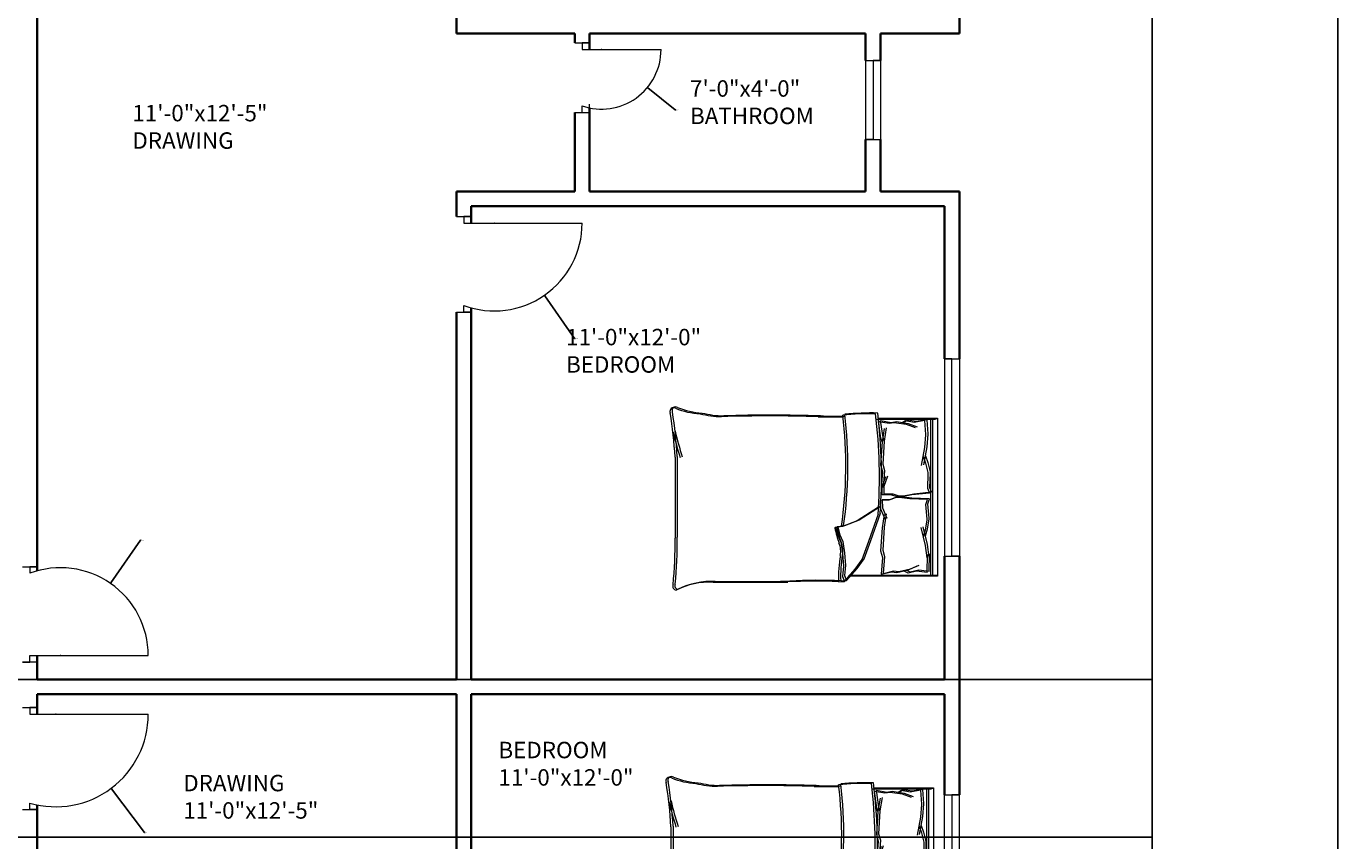
# Model space of a CAD drawing. Units: inches. Extents: x 2163 to 2982, y 1024 to 2288.
# Tile 19 of 22: x 2583 to 2982, y 1637 to 1885. Entities that reach past the tile are written whole.
import ezdxf

# ---------------------------------------------------------------- set-up
doc = ezdxf.new("R2010")
doc.units = ezdxf.units.IN
for name, color, linetype, lineweight in [('A-ANNO-DIMS', 2, 'Continuous', 18), ('A-ANNO-TTLB', 7, 'Continuous', 25), ('A-AREA-IDEN', 7, 'Continuous', 18), ('A-DOOR', 11, 'Continuous', 18), ('A-FURN', 8, 'Continuous', 13), ('A-GLAZ', 161, 'Continuous', 18), ('A-WALL', 7, 'Continuous', 35)]:
    doc.layers.add(name, color=color, linetype=linetype, lineweight=lineweight)
doc.styles.get("Standard").update_dxf_attribs({"font": 'arial.ttf'})
doc.dimstyles.get("Standard").update_dxf_attribs({"dimtxt": 0.18, "dimasz": 0.18, "dimexe": 0.18, "dimexo": 0.0625, "dimgap": 0.09, "dimtad": 0, "dimtih": 1, "dimtoh": 1, "dimdec": 4, "dimzin": 0, "dimdsep": 46, "dimtxsty": 'Standard', "dimcen": 0.09, "dimadec": 0, "dimazin": 0, "dimtfac": 1, "dimtdec": 4, "dimtofl": 0, "dimtmove": 0, "dimatfit": 3, "dimfxl": 1, "dimtolj": 1, "dimtzin": 0, "dimarcsym": 0})

# ---------------------------------------------------------------- blocks, each defined once
blk = doc.blocks.new('BED-DOUBLE')
for p, q in [((27.75, 52.87), (24.5, 49.16)), ((27.75, 52.87), (24.5, 49.16)), ((28.38, 53.1), (25.13, 49.39)), ((28.38, 53.1), (25.13, 49.39)), ((29.49, 52.95), (27.75, 52.87, 3.87)), ((29.49, 52.95), (27.75, 52.87, 3.87)), ((28.36, 51.33), (27.75, 52.87)), ((28.36, 51.33), (27.75, 52.87)), ((30.13, 53.18), (28.38, 53.1, 3.87)), ((29, 51.56), (28.38, 53.1)), ((30.13, 53.18), (28.38, 53.1, 3.87)), ((29, 51.56), (28.38, 53.1)), ((0, 51.49), (0.64, 51.49)), ((0, 3.47), (0, 51.49)), ((0, 51.27), (26.61, 51.27)), ((0, 51.27), (26.61, 51.27)), ((0.64, 51.49), (27.25, 51.49)), ((0.64, 51.49), (27.25, 51.49)), ((1.53, 3.48), (1.53, 51.27)), ((1.53, 3.47), (1.53, 51.27)), ((2.17, 3.7), (2.17, 51.49)), ((2.17, 3.7), (2.17, 51.49)), ((2.56, 50.11), (2.46, 44.71)), ((2.56, 50.11), (2.46, 44.71)), ((2.56, 50.11), (5.77, 49.73)), ((2.56, 50.11), (5.77, 49.73)), ((3.2, 50.34), (3.1, 44.94)), ((3.2, 50.34), (3.1, 44.94)), ((3.2, 50.34), (6.41, 49.96)), ((3.2, 50.34), (6.41, 49.96)), ((8.26, 49.31), (5.58, 48.13)), ((8.26, 49.31), (5.58, 48.13)), ((5.77, 49.73), (8.34, 50.33)), ((5.77, 49.73), (8.34, 50.33)), ((8.9, 49.54), (6.22, 48.36)), ((8.9, 49.54), (6.22, 48.36)), ((6.41, 49.96), (8.98, 50.56)), ((6.41, 49.96), (8.98, 50.56)), ((11.83, 50.11), (8.26, 49.31)), ((11.83, 50.11), (8.26, 49.31)), ((8.34, 50.33), (9.38, 49.81)), ((8.34, 50.33), (9.38, 49.81)), ((12.47, 50.34), (8.9, 49.54)), ((12.47, 50.34), (8.9, 49.54)), ((8.98, 50.56), (10.02, 50.04)), ((8.98, 50.56), (10.02, 50.04)), ((13.43, 49.92), (11.83, 50.11)), ((13.43, 49.92), (11.83, 50.11)), ((14.07, 50.15), (12.47, 50.34)), ((14.07, 50.15), (12.47, 50.34)), ((16.57, 50.7), (13.43, 49.92)), ((16.57, 50.7), (13.43, 49.92)), ((17.21, 50.93), (14.07, 50.15)), ((17.21, 50.93), (14.07, 50.15)), ((16.17, 45.57), (16.57, 50.7)), ((16.17, 45.57), (16.57, 50.7)), ((16.81, 45.79), (17.21, 50.93)), ((16.81, 45.79), (17.21, 50.93)), ((24.5, 49.16), (22.33, 46.22)), ((24.5, 49.16), (22.33, 46.22)), ((25.13, 49.39), (22.97, 46.45)), ((25.13, 49.39), (22.97, 46.45)), ((28.06, 48.23), (28.36, 51.33)), ((28.06, 48.23), (28.36, 51.33)), ((28.36, 44.36), (28.06, 48.23)), ((28.36, 44.36), (28.06, 48.23)), ((28.69, 48.46), (29, 51.56)), ((28.69, 48.46), (29, 51.56)), ((29, 44.59), (28.69, 48.46)), ((29, 44.59), (28.69, 48.46)), ((2.46, 44.71), (2.54, 45.71)), ((2.46, 44.71), (2.54, 45.71)), ((2.54, 45.71), (3.07, 41.91)), ((2.54, 45.71), (3.07, 41.91)), ((3.1, 44.94), (3.18, 45.94)), ((3.1, 44.94), (3.18, 45.94)), ((3.18, 45.94), (3.71, 42.14)), ((3.18, 45.94), (3.71, 42.14)), ((16.73, 43.61), (16.17, 45.57)), ((16.73, 43.61), (16.17, 45.57)), ((17.37, 43.83), (16.81, 45.79)), ((17.37, 43.83), (16.81, 45.79)), ((22.33, 46.22), (20.32, 40.64)), ((22.33, 46.22), (20.32, 40.64)), ((22.97, 46.45), (20.96, 40.87)), ((22.97, 46.45), (20.96, 40.87)), ((28.83, 40.95), (28.36, 44.36)), ((28.83, 40.95), (28.36, 44.36)), ((29.47, 41.18), (29, 44.59)), ((29.47, 41.18), (29, 44.59)), ((3.07, 41.91), (4.42, 36.49)), ((3.07, 41.91), (4.42, 36.49)), ((3.71, 42.14), (5.06, 36.72)), ((3.71, 42.14), (5.06, 36.72)), ((16.29, 36.6), (16.73, 43.61)), ((16.29, 36.6), (16.73, 43.61)), ((16.93, 36.82), (17.37, 43.83)), ((16.93, 36.82), (17.37, 43.83)), ((20.32, 40.64), (17.38, 32.31)), ((20.32, 40.64), (17.38, 32.31)), ((20.96, 40.87), (18.02, 32.53)), ((20.96, 40.87), (18.02, 32.53)), ((29.76, 38.94), (28.83, 40.95)), ((29.76, 38.94), (28.83, 40.95)), ((30.4, 39.17), (29.47, 41.18)), ((30.4, 39.17), (29.47, 41.18)), ((79.88, 15.29), (79.88, 39.91)), ((79.88, 15.29), (79.88, 39.91)), ((3.08, 37.14), (2.54, 34.2)), ((3.08, 37.13), (2.54, 34.2)), ((3.67, 39.2), (3.08, 37.14)), ((3.67, 39.2), (3.08, 37.13)), ((3.72, 37.36), (3.18, 34.43)), ((3.72, 37.36), (3.18, 34.43)), ((4.31, 39.43), (3.72, 37.36)), ((4.31, 39.43), (3.72, 37.36)), ((15.63, 32.56), (16.29, 36.6)), ((15.63, 32.56), (16.29, 36.6)), ((16.27, 32.79), (16.93, 36.82)), ((16.27, 32.79), (16.93, 36.82)), ((23.88, 34.45), (28.36, 36.15)), ((23.88, 34.45), (28.36, 36.15)), ((24.52, 34.68), (29, 36.38)), ((24.52, 34.68), (29, 36.38)), ((28.36, 36.15), (30.38, 36.46)), ((28.36, 36.15), (30.38, 36.46)), ((29, 36.38), (31.02, 36.69)), ((29, 36.38), (31.02, 36.69)), ((30.38, 36.46), (29.76, 38.94)), ((30.38, 36.46), (29.76, 38.94)), ((31.02, 36.69), (30.4, 39.17)), ((31.02, 36.69), (30.4, 39.17)), ((79.24, 15.06), (79.24, 39.68)), ((79.24, 15.06), (79.24, 39.68)), ((2.54, 34.2), (2.56, 33.88)), ((2.54, 34.2), (2.56, 33.88)), ((2.56, 33.88), (2.98, 29.46)), ((2.56, 33.88), (2.98, 29.46)), ((3.18, 34.43), (3.2, 34.11)), ((3.18, 34.43), (3.2, 34.11)), ((3.2, 34.11), (3.62, 29.68)), ((3.2, 34.11), (3.62, 29.68)), ((16.74, 30.75), (15.45, 33.82)), ((16.74, 30.75), (15.45, 33.82)), ((17.38, 30.98), (16.09, 34.05)), ((17.38, 30.98), (16.09, 34.05)), ((17.38, 30.26), (23.88, 34.45)), ((17.38, 30.26), (23.88, 34.45)), ((18.02, 30.49), (24.52, 34.68)), ((18.02, 30.49), (24.52, 34.68)), ((2.98, 29.46), (2.49, 27.98)), ((2.98, 29.46), (2.49, 27.98)), ((2.49, 27.98), (7.87, 27.73)), ((2.49, 27.98), (7.87, 27.73)), ((3.62, 29.68), (3.13, 28.21)), ((3.62, 29.68), (3.13, 28.2)), ((3.13, 28.21), (8.51, 27.96)), ((3.13, 28.2), (8.51, 27.96)), ((8.51, 27.96), (11.72, 27.58)), ((8.51, 27.96), (11.72, 27.58)), ((12.38, 27.44), (14.22, 28.13)), ((12.38, 27.44), (14.22, 28.13)), ((13.02, 27.66), (14.86, 28.36)), ((13.02, 27.66), (14.86, 28.36)), ((14.22, 28.13), (16.89, 28.3)), ((14.22, 28.13), (16.89, 28.3)), ((14.86, 28.36), (17.53, 28.53)), ((14.86, 28.36), (17.53, 28.53)), ((16.89, 28.3), (16.74, 30.75)), ((16.89, 28.3), (16.74, 30.75)), ((17.53, 28.53), (17.38, 30.98)), ((17.53, 28.53), (17.38, 30.98)), ((1.87, 25.98), (7.22, 26.56)), ((1.87, 25.98), (7.22, 26.56)), ((2.45, 24.54), (1.87, 25.98)), ((2.45, 24.54), (1.87, 25.98)), ((2.3, 20.09), (2.45, 24.54)), ((2.3, 20.09), (2.45, 24.54)), ((2.51, 26.21), (7.86, 26.79)), ((2.51, 26.21), (7.86, 26.79)), ((3.09, 24.77), (2.51, 26.21)), ((3.09, 24.77), (2.51, 26.21)), ((2.94, 20.32), (3.09, 24.77)), ((2.94, 20.32), (3.09, 24.77)), ((7.22, 26.56), (10.4, 27.14)), ((7.22, 26.56), (10.4, 27.14)), ((7.86, 26.79), (11.04, 27.37)), ((7.86, 26.79), (11.04, 27.37)), ((7.87, 27.73), (11.08, 27.35)), ((7.87, 27.73), (11.08, 27.35)), ((10.4, 27.14), (11.7, 27.14)), ((10.4, 27.14), (11.7, 27.14)), ((11.04, 27.37), (12.34, 27.37)), ((11.04, 27.37), (12.34, 27.37)), ((11.08, 27.35), (12.38, 27.44)), ((11.08, 27.35), (12.38, 27.44)), ((11.7, 27.14), (13.58, 26.56)), ((11.7, 27.14), (13.58, 26.56)), ((11.72, 27.58), (13.02, 27.66)), ((11.72, 27.58), (13.02, 27.66)), ((12.34, 27.37), (14.22, 26.79)), ((12.34, 27.37), (14.22, 26.79)), ((13.58, 26.56), (16.26, 26.56)), ((13.58, 26.56), (16.26, 26.56)), ((14.22, 26.79), (16.9, 26.79)), ((14.22, 26.79), (16.9, 26.79)), ((16.26, 24.1), (15.17, 20.96)), ((16.26, 24.1), (15.17, 20.96)), ((16.9, 24.33), (15.81, 21.19)), ((16.9, 24.33), (15.81, 21.19)), ((16.17, 19.38), (16.57, 24.52)), ((16.17, 19.38), (16.57, 24.52)), ((16.26, 26.56), (16.26, 24.1)), ((16.26, 26.56), (16.26, 24.1)), ((16.81, 19.61), (17.21, 24.74)), ((16.81, 19.61), (17.21, 24.74)), ((16.9, 26.79), (16.9, 24.33)), ((16.9, 26.79), (16.9, 24.33)), ((2.3, 19.77), (2.3, 20.09)), ((2.3, 19.77), (2.3, 20.09)), ((2.94, 20), (2.94, 20.32)), ((2.94, 20), (2.94, 20.32)), ((3.67, 17.11), (2.94, 20)), ((3.67, 17.11), (2.94, 20)), ((3.03, 16.88), (2.3, 19.77)), ((3.03, 16.88), (2.3, 19.77)), ((3.75, 14.85), (3.03, 16.88)), ((3.75, 14.85), (3.03, 16.88)), ((3.32, 12.11), (4.33, 17.6)), ((3.32, 12.11), (4.33, 17.6)), ((4.39, 15.08), (3.67, 17.11)), ((4.39, 15.08), (3.67, 17.11)), ((3.96, 12.34), (4.97, 17.83)), ((3.96, 12.34), (4.97, 17.83)), ((16.73, 17.42), (16.17, 19.38)), ((16.73, 17.42), (16.17, 19.38)), ((16.29, 10.41), (16.73, 17.42)), ((16.29, 10.41), (16.73, 17.42)), ((17.37, 17.65), (16.81, 19.61)), ((17.37, 17.65), (16.81, 19.61)), ((16.93, 10.64), (17.37, 17.65)), ((16.93, 10.64), (17.37, 17.65)), ((3.03, 8.28), (3.32, 12.11)), ((3.03, 8.28), (3.32, 12.11)), ((3.67, 8.51), (3.96, 12.34)), ((3.67, 8.51), (3.96, 12.34)), ((3.01, 8.18), (3.03, 8.28)), ((3.01, 8.18), (3.03, 8.28)), ((3.34, 3.9), (3.01, 8.18)), ((3.34, 3.9), (3.01, 8.18)), ((3.65, 8.41), (3.67, 8.51)), ((3.65, 8.41), (3.67, 8.51)), ((3.98, 4.13), (3.65, 8.41)), ((3.98, 4.13), (3.65, 8.41)), ((15.63, 6.38), (16.29, 10.41)), ((15.63, 6.38), (16.29, 10.41)), ((16.27, 6.61), (16.93, 10.64)), ((16.27, 6.61), (16.93, 10.64)), ((16.29, 10.41), (16.62, 9.28)), ((16.29, 10.41), (16.62, 9.28)), ((16.62, 9.28), (17.34, 4.18)), ((16.62, 9.28), (17.34, 4.18)), ((16.93, 10.64), (17.26, 9.51)), ((16.93, 10.64), (17.26, 9.51)), ((17.26, 9.51), (17.98, 4.41)), ((17.26, 9.51), (17.98, 4.41)), ((3.32, 3.89), (6.5, 4.47)), ((3.32, 3.89), (6.5, 4.47)), ((3.96, 4.12), (7.14, 4.7)), ((3.96, 4.12), (7.14, 4.7)), ((8.95, 5.05), (6.21, 6.06)), ((8.95, 5.05), (6.21, 6.06)), ((6.5, 4.47), (9.1, 4.04)), ((6.5, 4.47), (9.1, 4.04)), ((9.59, 5.28), (6.85, 6.29)), ((9.59, 5.28), (6.85, 6.29)), ((7.14, 4.7), (9.74, 4.27)), ((7.14, 4.7), (9.74, 4.27)), ((12.57, 4.47), (8.95, 5.05)), ((12.57, 4.47), (8.95, 5.05)), ((9.1, 4.04), (10.11, 4.62)), ((9.1, 4.04), (10.11, 4.62)), ((13.21, 4.7), (9.59, 5.28)), ((13.21, 4.7), (9.59, 5.28)), ((9.74, 4.27), (10.75, 4.85)), ((9.74, 4.27), (10.75, 4.85)), ((14.16, 4.76), (12.57, 4.47)), ((14.16, 4.76), (12.57, 4.47)), ((14.8, 4.99), (13.21, 4.7)), ((14.8, 4.99), (13.21, 4.7)), ((17.34, 4.18), (14.16, 4.76)), ((17.34, 4.18), (14.16, 4.76)), ((17.98, 4.41), (14.8, 4.99)), ((17.98, 4.41), (14.8, 4.99)), ((18.11, 3.48), (0, 3.48)), ((18.11, 3.47), (0, 3.47)), ((18.75, 3.7), (0.64, 3.7)), ((18.75, 3.7), (0.64, 3.7))]:
    blk.add_line(p, q)
for centre, radius, start, end in [((-6.66, 51.33), 36.18, 349.8763, 2.5657), ((-6.66, 51.33), 36.18, 349.8763, 2.5657), ((36.31, 182.27), 129.5, 266.9791, 273.8365), ((36.31, 182.27), 129.5, 266.9791, 273.8365), ((-6.02, 51.56), 36.18, 349.8763, 2.5657), ((-6.02, 51.56), 36.18, 349.8763, 2.5657), ((36.95, 182.49), 129.5, 266.9791, 273.8365), ((36.95, 182.49), 129.5, 266.9791, 273.8365), ((67.82, -4508.74), 4561.86, 90.00217, 90.28689), ((67.82, -4508.74), 4561.86, 90.00217, 90.28689), ((68.46, -4508.52), 4561.86, 90.00217, 90.28689), ((68.46, -4508.52), 4561.86, 90.00217, 90.28689), ((68.67, 76.16), 23.07, 267.4714, 296.4681), ((68.67, 76.16), 23.07, 267.4714, 296.4681), ((69.31, 76.39), 23.07, 267.4714, 296.4681), ((69.31, 76.39), 23.07, 267.4714, 296.4681), ((78.87, 54.41), 1.1, 332.6588, 86.02), ((78.87, 54.41), 1.1, 332.6588, 86.02), ((212.28, 41.15), 133.04, 174.4998, 180.6351), ((212.28, 41.15), 133.04, 174.4998, 180.6351), ((79.51, 54.64), 1.1, 332.6588, 86.02), ((79.51, 54.64), 1.1, 332.6588, 86.02), ((212.92, 41.38), 133.04, 174.4998, 180.6351), ((212.92, 41.38), 133.04, 174.4998, 180.6351), ((35.07, 43.74), 6.22, 168.6608, 203.7384), ((35.07, 43.74), 6.22, 168.6608, 203.7384), ((35.71, 43.97), 6.22, 168.6608, 203.7384), ((35.71, 43.97), 6.22, 168.6608, 203.7384), ((1.48, 31.15), 29.65, 10.6617, 19.8806), ((1.48, 31.15), 29.65, 10.6617, 19.8806), ((2.12, 31.38), 29.65, 10.6617, 19.8806), ((2.12, 31.38), 29.65, 10.6617, 19.8806), ((156.32, 17.76), 129.02, 171.7845, 186.9006), ((156.32, 17.76), 129.02, 171.7845, 186.9006), ((156.96, 17.98), 129.02, 171.7845, 186.9006), ((156.96, 17.98), 129.02, 171.7845, 186.9006), ((30.44, 36.64), 0.185, 250.2464, 1.1377), ((30.44, 36.64), 0.185, 250.2464, 1.1377), ((31.08, 36.86), 0.185, 250.2464, 1.1377), ((31.08, 36.86), 0.185, 250.2464, 1.1377), ((182.05, 21.36), 164.97, 176.0865, 186.7821), ((182.05, 21.36), 164.97, 176.0865, 186.7821), ((182.69, 21.59), 164.97, 176.0865, 186.7821), ((182.69, 21.59), 164.97, 176.0865, 186.7821), ((-23.71, -17.22), 106.46, 13.3832, 17.7053), ((-23.71, -17.22), 106.46, 13.3832, 17.7053), ((-23.07, -16.99), 106.46, 13.3832, 17.7053), ((-23.07, -16.99), 106.46, 13.3832, 17.7053), ((200.84, 21.43), 121.76, 182.9958, 189.4091), ((200.84, 21.43), 121.76, 182.9958, 189.4091), ((201.48, 21.66), 121.76, 182.9958, 189.4091), ((201.48, 21.65), 121.76, 182.9958, 189.4091), ((20.1, 85.16), 83.31, 268.7218, 275.604), ((20.1, 85.16), 83.31, 268.7218, 275.604), ((20.74, 85.39), 83.31, 268.7218, 275.604), ((20.74, 85.39), 83.31, 268.7218, 275.604), ((31.17, -167.31), 170.11, 88.4762, 91.0082), ((31.17, -167.31), 170.11, 88.4762, 91.0082), ((31.81, -167.08), 170.11, 88.4762, 91.0082), ((31.81, -167.08), 170.11, 88.4762, 91.0082), ((50.61, 484.82), 482.31, 268.2277, 271.7185), ((50.61, 484.82), 482.31, 268.2277, 271.7185), ((51.25, 485.05), 482.31, 268.2277, 271.7185), ((51.25, 485.05), 482.31, 268.2277, 271.7185), ((64.51, -26.9), 29.63, 76.0648, 88.9113), ((64.51, -26.9), 29.63, 76.0648, 88.9113), ((65.15, -26.67), 29.63, 76.0648, 88.9113), ((65.15, -26.67), 29.63, 76.0648, 88.9113), ((70.28, -21.66), 23.56, 67.9751, 86.652), ((70.28, -21.66), 23.56, 67.9751, 86.652), ((70.91, -21.43), 23.56, 67.9751, 86.652), ((70.91, -21.43), 23.56, 67.9751, 86.652), ((79.72, 1.09), 1.09, 236.1736, 23.4781), ((79.72, 1.09), 1.09, 236.1736, 23.4781), ((80.36, 1.32), 1.09, 236.1736, 23.4781), ((80.36, 1.32), 1.09, 236.1736, 23.4781)]:
    blk.add_arc(centre, radius, start, end)
blk = doc.blocks.new('WIN-24')
for p, q in [((0, 24), (4.5, 24)), ((0, 24), (0, 0)), ((4.5, 24), (2.25, 24)), ((2.25, 24), (2.25, 0)), ((4.5, 24), (4.5, 0)), ((2.25, 0), (0, 0)), ((0, 0), (4.5, 0))]:
    blk.add_line(p, q)
blk = doc.blocks.new('WIN-60')
for p, q in [((2.25, 60), (0, 60)), ((0, 60), (4.5, 60)), ((0, 60), (0, 0)), ((2.25, 0), (2.25, 60)), ((4.5, 60), (4.5, 0)), ((0, 0), (4.5, 0)), ((4.5, 0), (2.25, 0))]:
    blk.add_line(p, q)
blk = doc.blocks.new('*D29')
at = {"layer": 'A-ANNO-DIMS', "color": 0, "lineweight": -2, "transparency": 16777216}
for p, q in [((2285.34, 1738.83), (2285.34, 2288.1)), ((2285.52, 2287.92), (2576.05, 2287.92)), ((2867.16, 2287.92), (2576.63, 2287.92)), ((2867.34, 2229.33), (2867.34, 2288.1))]:
    blk.add_line(p, q, dxfattribs=at)
at = {"layer": 'A-ANNO-DIMS', "color": 0, "transparency": 16777216}
for points in [[(2285.52, 2287.95), (2285.52, 2287.89), (2285.34, 2287.92)], [(2867.16, 2287.95), (2867.16, 2287.89), (2867.34, 2287.92)]]:
    blk.add_solid(points, dxfattribs=at)
at = {"layer": 'Defpoints', "color": 0, "transparency": 16777216}
for p in [(2867.34, 2287.92), (2867.34, 2229.27), (2285.34, 1738.77)]:
    blk.add_point(p, dxfattribs=at)
at = {"layer": 'A-ANNO-DIMS', "color": 0, "transparency": 16777216, "insert": (2576.34, 2287.92), "char_height": 0.18, "attachment_point": 5}
blk.add_mtext('\\A1;582', dxfattribs=at)
blk = doc.blocks.new('*D31')
at = {"layer": 'A-ANNO-DIMS', "color": 0, "lineweight": -2, "transparency": 16777216}
for p, q in [((2867.4, 2229.27), (2926.17, 2229.27)), ((2925.99, 2229.09), (2925.99, 1957.95)), ((2925.99, 1686.45), (2925.99, 1957.59)), ((2862.9, 1686.27), (2926.17, 1686.27))]:
    blk.add_line(p, q, dxfattribs=at)
at = {"layer": 'A-ANNO-DIMS', "color": 0, "transparency": 16777216}
for points in [[(2925.96, 2229.09), (2926.02, 2229.09), (2925.99, 2229.27)], [(2925.96, 1686.45), (2926.02, 1686.45), (2925.99, 1686.27)]]:
    blk.add_solid(points, dxfattribs=at)
at = {"layer": 'Defpoints', "color": 0, "transparency": 16777216}
for p in [(2867.34, 2229.27), (2925.99, 2229.27), (2862.84, 1686.27)]:
    blk.add_point(p, dxfattribs=at)
at = {"layer": 'A-ANNO-DIMS', "color": 0, "transparency": 16777216, "insert": (2925.99, 1957.77), "char_height": 0.18, "attachment_point": 5}
blk.add_mtext('\\A1;543', dxfattribs=at)
blk = doc.blocks.new('*D32')
at = {"layer": 'A-ANNO-DIMS', "color": 0, "lineweight": -2, "transparency": 16777216}
for p, q in [((2867.4, 2229.27), (2926.17, 2229.27)), ((2925.99, 2229.09), (2925.99, 1686.35)), ((2925.99, 1143.25), (2925.99, 1685.99)), ((2867.4, 1143.07), (2926.17, 1143.07))]:
    blk.add_line(p, q, dxfattribs=at)
at = {"layer": 'A-ANNO-DIMS', "color": 0, "transparency": 16777216}
for points in [[(2925.96, 2229.09), (2926.02, 2229.09), (2925.99, 2229.27)], [(2925.96, 1143.25), (2926.02, 1143.25), (2925.99, 1143.07)]]:
    blk.add_solid(points, dxfattribs=at)
at = {"layer": 'Defpoints', "color": 0, "transparency": 16777216}
for p in [(2867.34, 2229.27), (2925.99, 2229.27), (2867.34, 1143.07)]:
    blk.add_point(p, dxfattribs=at)
at = {"layer": 'A-ANNO-DIMS', "color": 0, "transparency": 16777216, "insert": (2925.99, 1686.17), "char_height": 0.18, "attachment_point": 5}
blk.add_mtext('\\A1;1086.2', dxfattribs=at)
blk = doc.blocks.new('*D39')
at = {"layer": 'A-ANNO-DIMS', "color": 0, "lineweight": -2, "transparency": 16777216}
for p, q in [((2425.51, 1686.27), (2926.17, 1686.27)), ((2925.99, 1686.09), (2925.99, 1662.45)), ((2925.99, 1638.45), (2925.99, 1662.09)), ((2425.51, 1638.27), (2926.17, 1638.27))]:
    blk.add_line(p, q, dxfattribs=at)
at = {"layer": 'A-ANNO-DIMS', "color": 0, "transparency": 16777216}
for points in [[(2925.96, 1686.09), (2926.02, 1686.09), (2925.99, 1686.27)], [(2925.96, 1638.45), (2926.02, 1638.45), (2925.99, 1638.27)]]:
    blk.add_solid(points, dxfattribs=at)
at = {"layer": 'Defpoints', "color": 0, "transparency": 16777216}
for p in [(2425.44, 1686.27), (2925.99, 1686.27), (2425.44, 1638.27)]:
    blk.add_point(p, dxfattribs=at)
at = {"layer": 'A-ANNO-DIMS', "color": 0, "transparency": 16777216, "insert": (2925.99, 1662.27), "char_height": 0.18, "attachment_point": 5}
blk.add_mtext('\\A1;48', dxfattribs=at)
blk = doc.blocks.new('*D44')
at = {"layer": 'A-ANNO-DIMS', "color": 0, "lineweight": -2, "transparency": 16777216}
for p, q in [((2592.35, 1675.65), (2592.53, 1675.65)), ((2592.44, 1675.56), (2592.44, 1675.74)), ((2619.49, 1639.63), (2609.45, 1653)), ((2619.67, 1639.63), (2619.49, 1639.63))]:
    blk.add_line(p, q, dxfattribs=at)
at = {"layer": 'A-ANNO-DIMS', "color": 0, "transparency": 16777216}
blk.add_solid([(2609.48, 1653.02), (2609.43, 1652.98), (2609.34, 1653.14)], dxfattribs=at)
at = {"layer": 'Defpoints', "color": 0, "transparency": 16777216}
for p in [(2592.44, 1675.65), (2609.34, 1653.14)]:
    blk.add_point(p, dxfattribs=at)
at = {"layer": 'A-ANNO-DIMS', "color": 0, "transparency": 16777216, "insert": (2620.22, 1639.63), "char_height": 0.18, "attachment_point": 5}
blk.add_mtext('\\A1;R28.154', dxfattribs=at)
blk = doc.blocks.new('*D50')
at = {"layer": 'A-ANNO-DIMS', "color": 0, "lineweight": -2, "transparency": 16777216}
for p, q in [((2725.78, 1825.1), (2725.96, 1825.1)), ((2725.87, 1825.01), (2725.87, 1825.19)), ((2750.29, 1790.01), (2741.24, 1803.02)), ((2750.47, 1790.01), (2750.29, 1790.01))]:
    blk.add_line(p, q, dxfattribs=at)
at = {"layer": 'A-ANNO-DIMS', "color": 0, "transparency": 16777216}
blk.add_solid([(2741.26, 1803.04), (2741.21, 1803.01), (2741.13, 1803.17)], dxfattribs=at)
at = {"layer": 'Defpoints', "color": 0, "transparency": 16777216}
for p in [(2725.87, 1825.1), (2741.13, 1803.17)]:
    blk.add_point(p, dxfattribs=at)
at = {"layer": 'A-ANNO-DIMS', "color": 0, "transparency": 16777216, "insert": (2750.95, 1790.01), "char_height": 0.18, "attachment_point": 5}
blk.add_mtext('\\A1;R26.72', dxfattribs=at)
blk = doc.blocks.new('*D51')
at = {"layer": 'A-ANNO-DIMS', "color": 0, "lineweight": -2, "transparency": 16777216}
for p, q in [((2618.27, 1728.6), (2609.23, 1715.6)), ((2618.45, 1728.6), (2618.27, 1728.6)), ((2593.8, 1693.53), (2593.98, 1693.53)), ((2593.89, 1693.44), (2593.89, 1693.62))]:
    blk.add_line(p, q, dxfattribs=at)
at = {"layer": 'A-ANNO-DIMS', "color": 0, "transparency": 16777216}
blk.add_solid([(2609.21, 1715.62), (2609.26, 1715.58), (2609.13, 1715.45)], dxfattribs=at)
at = {"layer": 'Defpoints', "color": 0, "transparency": 16777216}
for p in [(2609.13, 1715.45), (2593.89, 1693.53)]:
    blk.add_point(p, dxfattribs=at)
at = {"layer": 'A-ANNO-DIMS', "color": 0, "transparency": 16777216, "insert": (2619, 1728.6), "char_height": 0.18, "attachment_point": 5}
blk.add_mtext('\\A1;R26.694', dxfattribs=at)
blk = doc.blocks.new('*D73')
at = {"layer": 'A-ANNO-DIMS', "color": 0, "lineweight": -2, "transparency": 16777216}
for p, q in [((2758.37, 1877.92), (2758.55, 1877.92)), ((2758.46, 1877.83), (2758.46, 1878.01)), ((2780.89, 1859.53), (2772.62, 1866.31)), ((2781.07, 1859.53), (2780.89, 1859.53))]:
    blk.add_line(p, q, dxfattribs=at)
at = {"layer": 'A-ANNO-DIMS', "color": 0, "transparency": 16777216}
blk.add_solid([(2772.64, 1866.34), (2772.6, 1866.29), (2772.48, 1866.43)], dxfattribs=at)
at = {"layer": 'Defpoints', "color": 0, "transparency": 16777216}
for p in [(2758.46, 1877.92), (2772.48, 1866.43)]:
    blk.add_point(p, dxfattribs=at)
at = {"layer": 'A-ANNO-DIMS', "color": 0, "transparency": 16777216, "insert": (2781.62, 1859.53), "char_height": 0.18, "attachment_point": 5}
blk.add_mtext('\\A1;R18.128', dxfattribs=at)

msp = doc.modelspace()

# ---------------------------------------------------------------- linework, layer by layer
at = {"layer": 'A-ANNO-TTLB'}
msp.add_lwpolyline([(2162.6841, 2274.6054), (2982.469, 2274.6054), (2982.469, 1045.9691), (2162.6841, 1045.9691)], close=True, dxfattribs=at)
at = {"layer": 'A-DOOR'}
for p, q in [((2750.3389, 1879.9188), (2754.8389, 1879.9188)), ((2754.8389, 1879.9188), (2752.5889, 1879.9188)), ((2752.5889, 1879.9188), (2752.5889, 1877.9188)), ((2752.5889, 1877.9188), (2776.5889, 1877.9188)), ((2752.5889, 1858.7688), (2752.5889, 1860.7688)), ((2754.8389, 1858.7688), (2754.8389, 1861.3385)), ((2750.3389, 1858.7688), (2754.8389, 1858.7688)), ((2714.3389, 1827.1014), (2718.8389, 1827.1014)), ((2718.8389, 1827.1014), (2716.5889, 1827.1014)), ((2716.5889, 1827.1014), (2716.5889, 1825.1014)), ((2716.5889, 1825.1014), (2752.5889, 1825.1014)), ((2716.5889, 1798.0467), (2716.5889, 1800.0467)), ((2714.3389, 1798.0467), (2718.8389, 1798.0467)), ((2718.8389, 1798.0467), (2716.5889, 1798.0467)), ((2582.3389, 1720.5499), (2586.8389, 1720.5499)), ((2586.8389, 1720.5499), (2584.5889, 1720.5499)), ((2584.5889, 1720.5499), (2584.5889, 1718.5499)), ((2584.5889, 1691.5305), (2584.5889, 1693.5305)), ((2584.5889, 1693.5305), (2620.5889, 1693.5305)), ((2586.8389, 1691.5305), (2582.3389, 1691.5305)), ((2582.3389, 1691.5305), (2584.5889, 1691.5305)), ((2582.3389, 1677.6524), (2586.8389, 1677.6524)), ((2586.8389, 1677.6524), (2584.5889, 1677.6524)), ((2584.5889, 1677.6524), (2584.5889, 1675.6524)), ((2584.5889, 1675.6524), (2620.5889, 1675.6524)), ((2584.5889, 1646.614), (2584.5889, 1648.614)), ((2582.3389, 1646.614), (2586.8389, 1646.614)), ((2586.8389, 1646.614), (2584.5889, 1646.614))]:
    msp.add_line(p, q, dxfattribs=at)
for centre, radius, start, end in [((2758.4614, 1877.9188), 18.1275, 251.097757, 360), ((2725.8704, 1825.1014), 26.7185, 249.672934, 360), ((2593.8949, 1693.5305), 26.694, 0, 110.402719), ((2592.4351, 1675.6524), 28.1538, 253.818042, 360)]:
    msp.add_arc(centre, radius, start, end, dxfattribs=at)
at = {"layer": 'A-WALL'}
for p, q in [((2586.8389, 2011.7688), (2586.8389, 1719.2751)), ((2714.3389, 1963.7688), (2714.3389, 1882.7688)), ((2867.3389, 1905.1374), (2867.3389, 1882.7688)), ((2714.3389, 1882.7688), (2750.3389, 1882.7688)), ((2750.3389, 1879.9188), (2750.3389, 1882.7688)), ((2838.8389, 1882.7688), (2754.8389, 1882.7688)), ((2754.8389, 1882.7688), (2754.8389, 1877.9188)), ((2754.8389, 1882.7688), (2838.8389, 1882.7688)), ((2838.8389, 1882.7688), (2838.8389, 1874.5615)), ((2867.3389, 1882.7688), (2843.3389, 1882.7688)), ((2843.3389, 1882.7688), (2862.8389, 1882.7688)), ((2843.3389, 1874.5615), (2843.3389, 1882.7688)), ((2754.8389, 1860.1569), (2754.8389, 1834.7688)), ((2750.3389, 1834.7688), (2750.3389, 1858.7688)), ((2838.8389, 1850.5615), (2838.8389, 1834.7688)), ((2843.3389, 1834.7688), (2843.3389, 1850.5615)), ((2714.3389, 1834.7688), (2750.3389, 1834.7688)), ((2714.3389, 1834.7688), (2714.3389, 1827.1014)), ((2754.8389, 1834.7688), (2838.8389, 1834.7688)), ((2843.3389, 1834.7688), (2867.3389, 1834.7688)), ((2867.3389, 1834.7688), (2867.3389, 1783.7638)), ((2718.8389, 1830.2688), (2862.8389, 1830.2688)), ((2718.8389, 1830.2688), (2718.8389, 1825.1014)), ((2862.8389, 1830.2688), (2862.8389, 1783.7638)), ((2714.3389, 1798.0467), (2714.3389, 1686.2688)), ((2718.8389, 1799.3247), (2718.8389, 1686.2688)), ((2862.8389, 1723.7638), (2862.8389, 1686.2688)), ((2867.3389, 1723.7638), (2867.3389, 1651.1733)), ((2586.8389, 1693.5305), (2586.8389, 1686.2688)), ((2586.8389, 1686.2688), (2714.3389, 1686.2688)), ((2718.8389, 1686.2688), (2862.8389, 1686.2688)), ((2586.8389, 1681.7688), (2714.3389, 1681.7688)), ((2586.8389, 1681.7688), (2586.8389, 1675.6524)), ((2714.3389, 1681.7688), (2714.3389, 1572.0744)), ((2718.8389, 1681.7688), (2718.8389, 1570.7042)), ((2718.8389, 1681.7688), (2862.8389, 1681.7688)), ((2862.8389, 1681.7688), (2862.8389, 1651.1733)), ((2586.8389, 1648.0603), (2586.8389, 1356.2688))]:
    msp.add_line(p, q, dxfattribs=at)

# ---------------------------------------------------------------- block references
at = {"layer": 'A-FURN', "rotation": 180}
for p in [(2860.7453, 1769.1724), (2859.4875, 1656.6782)]:
    msp.add_blockref('BED-DOUBLE', p, dxfattribs=at)
at = {"layer": 'A-GLAZ'}
for name, p in [('WIN-24', (2838.839, 1850.562)), ('WIN-60', (2862.839, 1723.7637))]:
    msp.add_blockref(name, p, dxfattribs=at)
at = {"layer": 'A-GLAZ', "extrusion": (0, 0, -1), "zscale": -1, "rotation": 180}
msp.add_blockref('WIN-60', (-2862.839, 1651.1734), dxfattribs=at)

# ---------------------------------------------------------------- texts
at = {"layer": 'A-AREA-IDEN', "char_height": 5, "attachment_point": 1}
for s, width, insert in [('7\'-0"x4\'-0"\\PBATHROOM', 37.624015, (2785.4074, 1868.576)), ('11\'-0"x12\'-5"\\PDRAWING', 86.750713, (2615.7616, 1861.0681)), ('11\'-0"x12\'-0"\\PBEDROOM', 49.776962, (2747.7027, 1792.9277)), ('BEDROOM\\P11\'-0"x12\'-0"', 60.332971, (2727.119, 1667.2605)), ('DRAWING\\P11\'-0"x12\'-5"', 69.474499, (2631.2335, 1657.2071))]:
    msp.add_mtext_dynamic_manual_height_columns(s, width=width, gutter_width=12.5, heights=[0], dxfattribs=dict(at, insert=insert))

# ---------------------------------------------------------------- dimensions: what is measured, and where the dimension line sits
at = {"layer": 'A-ANNO-DIMS'}
dim = msp.add_linear_dim(base=(2867.3389, 2287.9188), p1=(2285.3389, 1738.7688), p2=(2867.3389, 2229.2688), dimstyle='Standard', override={"dimdec": 0, "dimlfac": 1, "dimrnd": 0, "dimzin": 0, "dimdsep": 46, "dimlunit": 2}, dxfattribs=at)
dim.commit()
dim.dimension.update_dxf_attribs({"geometry": '*D29', "text_midpoint": (2576.3389, 2287.9188)})
for base, p1, p2, override, picture, middle in [((2925.9889, 2229.2688), (2862.8389, 1686.2688), (2867.3389, 2229.2688), {"dimdec": 0, "dimlfac": 1, "dimrnd": 0, "dimzin": 0, "dimdsep": 46, "dimlunit": 2}, '*D31', (2925.9889, 1957.7688)), ((2925.9889, 2229.2688), (2867.3389, 1143.0732), (2867.3389, 2229.2688), {"dimdec": 1, "dimlfac": 1, "dimrnd": 0, "dimzin": 0, "dimdsep": 46, "dimlunit": 2}, '*D32', (2925.9889, 1686.171)), ((2925.9889, 1686.2688), (2425.4434, 1638.2688), (2425.4434, 1686.2688), {"dimdec": 0, "dimlfac": 1, "dimrnd": 0, "dimzin": 0, "dimdsep": 46, "dimlunit": 2}, '*D39', (2925.9889, 1662.2688))]:
    dim = msp.add_linear_dim(base=base, p1=p1, p2=p2, angle=90, dimstyle='Standard', override=override, dxfattribs=at)
    dim.commit()
    dim.dimension.update_dxf_attribs({"geometry": picture, "text_midpoint": middle})
for center, mpoint, override, picture, middle in [((2758.4614, 1877.9188), (2772.4802, 1866.4262), {"dimdec": 3, "dimlfac": 1, "dimrnd": 0, "dimzin": 0, "dimdsep": 46, "dimlunit": 2}, '*D73', (2781.6214, 1859.5306)), ((2725.8704, 1825.1014), (2741.1329, 1803.1711), {"dimdec": 2, "dimlfac": 1, "dimrnd": 0, "dimzin": 0, "dimdsep": 46, "dimlunit": 2}, '*D50', (2750.9493, 1790.013)), ((2593.8949, 1693.5305), (2609.1288, 1715.4508), {"dimdec": 3, "dimlfac": 1, "dimrnd": 0, "dimzin": 0, "dimdsep": 46, "dimlunit": 2}, '*D51', (2618.9986, 1728.6029)), ((2592.4351, 1675.6524), (2609.343, 1653.141), {"dimdec": 3, "dimlfac": 1, "dimrnd": 0, "dimzin": 0, "dimdsep": 46, "dimlunit": 2}, '*D44', (2620.2171, 1639.6342))]:
    dim = msp.add_radius_dim(center=center, mpoint=mpoint, dimstyle='Standard', override=override, dxfattribs=at)
    dim.commit()
    dim.dimension.update_dxf_attribs({"geometry": picture, "text_midpoint": middle, "dimtype": 164})

doc.saveas('drawing.dxf')
